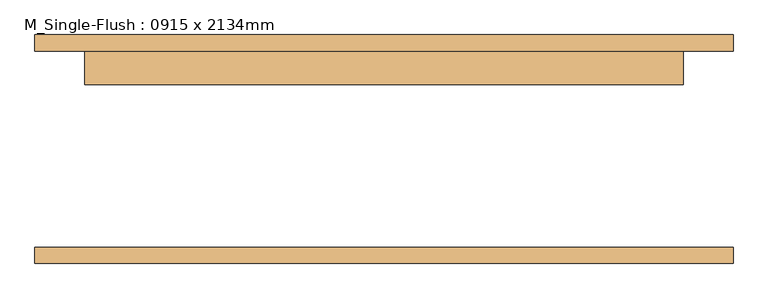
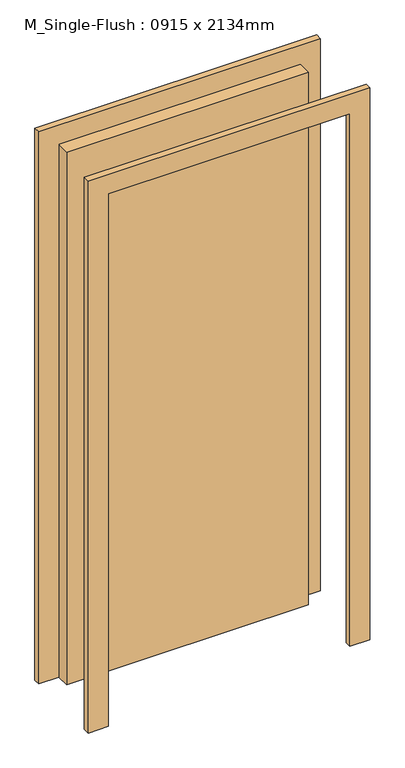
"""IFC4 building model written with IfcOpenShell, lengths in millimetres: door geometry, M_Single-Flush : 0915 x 2134mm."""

from ifc_helpers import new_model, si_unit, frame, origin, origin_with_axes, place, context, project, spatial, polyline, outline, extrude, source, transform, mapped, element, save


def m_single_flush_0915_x_2134mm_9cebaac8(model_context):
    return source(origin(), model_context, "Body", "SweptSolid", [
        extrude(outline(polyline([(2210.0, -533.5), (0.0, -533.5), (0.0, -457.5), (2134.0, -457.5), (2134.0, 457.5), (0.0, 457.5), (0.0, 533.5), (2210.0, 533.5), (2210.0, -533.5)])), frame((0.0, 150.0, 0.0), z_axis=(0.0, 1.0, 0.0), x_axis=(0.0, 0.0, 1.0)), (0.0, 0.0, 1.0), 25.0),
        extrude(outline(polyline([(2210.0, 533.5), (2210.0, -533.5), (0.0, -533.5), (0.0, -457.5), (2134.0, -457.5), (2134.0, 457.5), (0.0, 457.5), (0.0, 533.5), (2210.0, 533.5)])), frame((0.0, -175.0, 0.0), z_axis=(0.0, 1.0, 0.0), x_axis=(0.0, 0.0, 1.0)), (0.0, 0.0, 1.0), 25.0),
        extrude(outline(polyline([(457.5, 99.0), (-457.5, 99.0), (-457.5, 150.0), (457.5, 150.0), (457.5, 99.0)])), origin_with_axes(), (0.0, 0.0, 1.0), 2134.0),
    ])


if __name__ == "__main__":
    model = new_model("IFC4")
    model_context = context("Model", 3, world=origin())
    ifc_project = project(units=[si_unit("LENGTHUNIT", "METRE", prefix="MILLI")], contexts=[model_context])
    site = spatial("IfcSite", under=ifc_project)
    building = spatial("IfcBuilding", under=site)
    placement = place(None, origin())
    m_single_flush_0915_x_2134mm_shape = m_single_flush_0915_x_2134mm_9cebaac8(model_context)
    element("IfcDoor", 1, ObjectType="M_Single-Flush : 0915 x 2134mm", at=placement, inside=building, context=model_context, shape_type="MappedRepresentation", body=[
        mapped(m_single_flush_0915_x_2134mm_shape, transform((0.0, 0.0, 0.0), x_axis=(1.0, 0.0, 0.0), y_axis=(0.0, 1.0, 0.0), z_axis=(0.0, 0.0, 1.0))),
    ])
    save(model, "model.ifc")

# Revit data of these elements
# Type "M_Single-Flush : 0915 x 2134mm"
#   Type Mark = "20"
#   Construction Type Id = "MDOOR"
#   Analytic Construction = "Metal"
#   Thickness = 51 mm
#   Thermal Resistance (R) = 0.270117 (m²·K)/W
#   Heat Transfer Coefficient (U) = 3.7021 W/(m²·K)
#   Height = 2134 mm
#   Trim Projection Ext = 25 mm
#   Trim Projection Int = 25 mm
#   Trim Width = 76 mm
#   Width = 915 mm
#   Define Thermal Properties by = 1
#   Define Thermal Properties by = 1
#   Door Material = Door - Panel
#   Frame Material = Door - Frame
#   Visual Light Transmittance = 0
#   Solar Heat Gain Coefficient = 0
#   Function = (empty or 0)
#   Wall Closure = (empty or 0)
# Element 1 (IfcDoor, "M_Single-Flush : 0915 x 2134mm")
#   Materials on its faces: "Door - Frame", "Door - Panel"
# Materials
#   "Door - Panel": class "Wood", colour RGB 210 159 95, transparency 0, Cost = 0
#   "Door - Frame": colour RGB 118 70 51, transparency 0, Cost = 0
